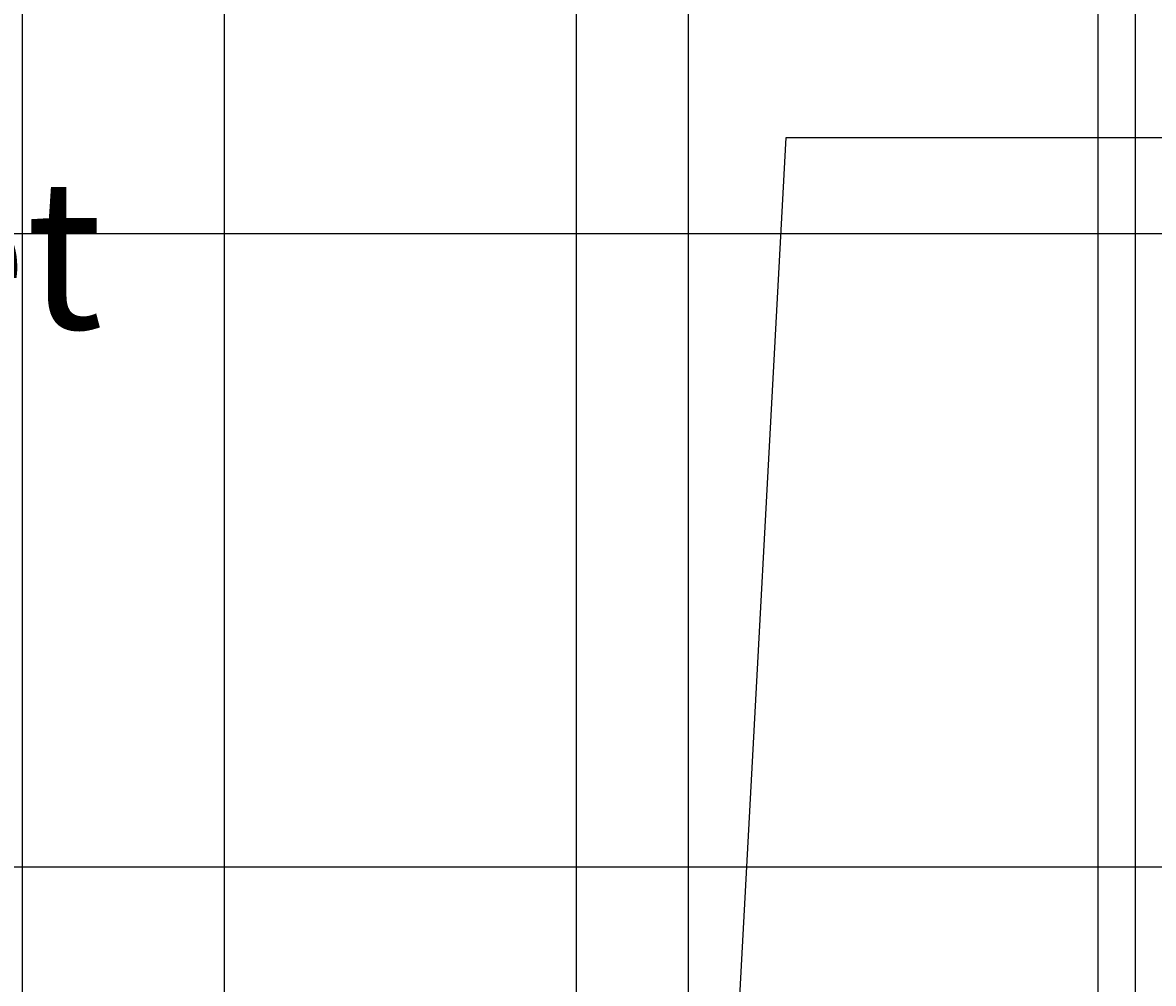
# Model space of a CAD drawing. Units: inches. Extents: x -12 to 334, y -10 to 186.
# Tile 25 of 77: x 58 to 88, y 135 to 160. Entities that reach past the tile are written whole.
import ezdxf
from ezdxf import colors
from ezdxf.entities.mleader import LeaderData, LeaderLine
from ezdxf.math import Vec2, Vec3

# ---------------------------------------------------------------- set-up
doc = ezdxf.new("R2010")
doc.units = ezdxf.units.IN
doc.header["$MEASUREMENT"] = 0
doc.layers.add('M-ANNO-TEXT', color=3, linetype='Continuous', lineweight=25)
doc.layers.add('M-DIMS', color=2, linetype='Continuous', lineweight=18)
doc.styles.get("Standard").update_dxf_attribs({"font": 'arial.ttf'})
doc.dimstyles.get("Standard").update_dxf_attribs({"dimtxt": 0.18, "dimasz": 0.18, "dimexe": 0.18, "dimexo": 0.0625, "dimgap": 0.09, "dimtad": 0, "dimtih": 1, "dimtoh": 1, "dimdec": 4, "dimzin": 0, "dimdsep": 46, "dimtxsty": 'Standard', "dimcen": 0.09, "dimadec": 0, "dimazin": 0, "dimtfac": 1, "dimtdec": 4, "dimtofl": 0, "dimtmove": 0, "dimatfit": 3, "dimfxl": 1, "dimtolj": 1, "dimtzin": 0, "dimarcsym": 0})

# ---------------------------------------------------------------- blocks, each defined once
blk = doc.blocks.new('*D3')
at = {"layer": 'Defpoints', "color": 0, "transparency": 16777216}
for p in [(58.1, 169.385), (32.1, 127.708), (58.1, 127.708)]:
    blk.add_point(p, dxfattribs=at)
at = {"layer": 'M-DIMS', "color": 0, "lineweight": -2, "transparency": 16777216}
for p, q in [((32.1, 127.77), (32.1, 169.565)), ((58.1, 127.77), (58.1, 169.565)), ((32.28, 169.385), (44.88, 169.385)), ((57.92, 169.385), (45.321, 169.385))]:
    blk.add_line(p, q, dxfattribs=at)
at = {"layer": 'M-DIMS', "color": 0, "transparency": 16777216}
for points in [[(32.28, 169.415), (32.28, 169.355), (32.1, 169.385)], [(57.92, 169.415), (57.92, 169.355), (58.1, 169.385)]]:
    blk.add_solid(points, dxfattribs=at)
at = {"layer": 'M-DIMS', "color": 0, "transparency": 16777216, "insert": (45.1, 169.385), "char_height": 0.18, "attachment_point": 5}
blk.add_mtext('\\A1;26', dxfattribs=at)
blk = doc.blocks.new('*D10')
at = {"layer": 'Defpoints', "color": 0, "transparency": 16777216}
for p in [(63.5, 169.385), (58.1, 127.708), (63.5, 109.058)]:
    blk.add_point(p, dxfattribs=at)
at = {"layer": 'M-DIMS', "color": 0, "lineweight": -2, "transparency": 16777216}
for p, q in [((58.1, 127.77), (58.1, 169.565)), ((63.5, 109.121), (63.5, 169.565)), ((58.28, 169.385), (60.547, 169.385)), ((63.32, 169.385), (61.054, 169.385))]:
    blk.add_line(p, q, dxfattribs=at)
at = {"layer": 'M-DIMS', "color": 0, "transparency": 16777216}
for points in [[(58.28, 169.415), (58.28, 169.355), (58.1, 169.385)], [(63.32, 169.415), (63.32, 169.355), (63.5, 169.385)]]:
    blk.add_solid(points, dxfattribs=at)
at = {"layer": 'M-DIMS', "color": 0, "transparency": 16777216, "insert": (60.8, 169.385), "char_height": 0.18, "attachment_point": 5}
blk.add_mtext('\\A1;5.4', dxfattribs=at)
blk = doc.blocks.new('*D11')
at = {"layer": 'Defpoints', "color": 0, "transparency": 16777216}
for p in [(72.924, 169.385), (63.5, 109.058), (72.924, 109.058)]:
    blk.add_point(p, dxfattribs=at)
at = {"layer": 'M-DIMS', "color": 0, "lineweight": -2, "transparency": 16777216}
for p, q in [((63.5, 109.121), (63.5, 169.565)), ((72.924, 109.121), (72.924, 169.565)), ((63.68, 169.385), (67.819, 169.385)), ((72.744, 169.385), (68.606, 169.385))]:
    blk.add_line(p, q, dxfattribs=at)
at = {"layer": 'M-DIMS', "color": 0, "transparency": 16777216}
for points in [[(63.68, 169.415), (63.68, 169.355), (63.5, 169.385)], [(72.744, 169.415), (72.744, 169.355), (72.924, 169.385)]]:
    blk.add_solid(points, dxfattribs=at)
at = {"layer": 'M-DIMS', "color": 0, "transparency": 16777216, "insert": (68.212, 169.385), "char_height": 0.18, "attachment_point": 5}
blk.add_mtext('\\A1;9.424', dxfattribs=at)
blk = doc.blocks.new('*D12')
at = {"layer": 'Defpoints', "color": 0, "transparency": 16777216}
for p in [(75.924, 169.385), (72.924, 109.058), (75.924, 109.058)]:
    blk.add_point(p, dxfattribs=at)
at = {"layer": 'M-DIMS', "color": 0, "lineweight": -2, "transparency": 16777216}
for p, q in [((72.924, 109.121), (72.924, 169.565)), ((75.924, 109.121), (75.924, 169.565)), ((73.104, 169.385), (74.275, 169.385)), ((75.744, 169.385), (74.573, 169.385))]:
    blk.add_line(p, q, dxfattribs=at)
at = {"layer": 'M-DIMS', "color": 0, "transparency": 16777216}
for points in [[(73.104, 169.415), (73.104, 169.355), (72.924, 169.385)], [(75.744, 169.415), (75.744, 169.355), (75.924, 169.385)]]:
    blk.add_solid(points, dxfattribs=at)
at = {"layer": 'M-DIMS', "color": 0, "transparency": 16777216, "insert": (74.424, 169.385), "char_height": 0.18, "attachment_point": 5}
blk.add_mtext('\\A1;3', dxfattribs=at)
blk = doc.blocks.new('*D13')
at = {"layer": 'Defpoints', "color": 0, "transparency": 16777216}
for p in [(86.888, 169.385), (75.924, 109.058), (86.888, 109.058)]:
    blk.add_point(p, dxfattribs=at)
at = {"layer": 'M-DIMS', "color": 0, "lineweight": -2, "transparency": 16777216}
for p, q in [((75.924, 109.121), (75.924, 169.565)), ((86.888, 109.121), (86.888, 169.565)), ((76.104, 169.385), (80.951, 169.385)), ((86.708, 169.385), (81.861, 169.385))]:
    blk.add_line(p, q, dxfattribs=at)
at = {"layer": 'M-DIMS', "color": 0, "transparency": 16777216}
for points in [[(76.104, 169.415), (76.104, 169.355), (75.924, 169.385)], [(86.708, 169.415), (86.708, 169.355), (86.888, 169.385)]]:
    blk.add_solid(points, dxfattribs=at)
at = {"layer": 'M-DIMS', "color": 0, "transparency": 16777216, "insert": (81.406, 169.385), "char_height": 0.18, "attachment_point": 5}
blk.add_mtext('\\A1;10.964', dxfattribs=at)
blk = doc.blocks.new('*D15')
at = {"layer": 'Defpoints', "color": 0, "transparency": 16777216}
for p in [(106.177, 169.385), (86.888, 109.058), (106.177, 102.896)]:
    blk.add_point(p, dxfattribs=at)
at = {"layer": 'M-DIMS', "color": 0, "lineweight": -2, "transparency": 16777216}
for p, q in [((86.888, 109.121), (86.888, 169.565)), ((106.177, 102.958), (106.177, 169.565)), ((87.068, 169.385), (96.147, 169.385)), ((105.997, 169.385), (96.918, 169.385))]:
    blk.add_line(p, q, dxfattribs=at)
at = {"layer": 'M-DIMS', "color": 0, "transparency": 16777216}
for points in [[(87.068, 169.415), (87.068, 169.355), (86.888, 169.385)], [(105.997, 169.415), (105.997, 169.355), (106.177, 169.385)]]:
    blk.add_solid(points, dxfattribs=at)
at = {"layer": 'M-DIMS', "color": 0, "transparency": 16777216, "insert": (96.532, 169.385), "char_height": 0.18, "attachment_point": 5}
blk.add_mtext('\\A1;19.29', dxfattribs=at)
blk = doc.blocks.new('*D22')
at = {"layer": 'Defpoints', "color": 0, "transparency": 16777216}
for p in [(190.342, 154.835), (-11.174, 137.887), (195.342, 137.887)]:
    blk.add_point(p, dxfattribs=at)
at = {"layer": 'M-DIMS', "color": 0, "lineweight": -2, "transparency": 16777216}
for p, q in [((190.28, 154.835), (-11.354, 154.835)), ((-11.174, 154.655), (-11.174, 146.543)), ((-11.174, 138.067), (-11.174, 146.179)), ((195.28, 137.887), (-11.354, 137.887))]:
    blk.add_line(p, q, dxfattribs=at)
at = {"layer": 'M-DIMS', "color": 0, "transparency": 16777216}
for points in [[(-11.204, 154.655), (-11.144, 154.655), (-11.174, 154.835)], [(-11.204, 138.067), (-11.144, 138.067), (-11.174, 137.887)]]:
    blk.add_solid(points, dxfattribs=at)
at = {"layer": 'M-DIMS', "color": 0, "transparency": 16777216, "insert": (-11.174, 146.361), "char_height": 0.18, "attachment_point": 5}
blk.add_mtext('\\A1;16.947', dxfattribs=at)
blk = doc.blocks.new('*D26')
at = {"layer": 'Defpoints', "color": 0, "transparency": 16777216}
for p in [(87.888, 169.385), (87.888, 56.321), (58.1, 33.675)]:
    blk.add_point(p, dxfattribs=at)
at = {"layer": 'M-DIMS', "color": 0, "lineweight": -2, "transparency": 16777216}
for p, q in [((58.1, 33.738), (58.1, 169.565)), ((87.888, 56.383), (87.888, 169.565)), ((58.28, 169.385), (72.599, 169.385)), ((87.708, 169.385), (73.389, 169.385))]:
    blk.add_line(p, q, dxfattribs=at)
at = {"layer": 'M-DIMS', "color": 0, "transparency": 16777216}
for points in [[(58.28, 169.415), (58.28, 169.355), (58.1, 169.385)], [(87.708, 169.415), (87.708, 169.355), (87.888, 169.385)]]:
    blk.add_solid(points, dxfattribs=at)
at = {"layer": 'M-DIMS', "color": 0, "transparency": 16777216, "insert": (72.994, 169.385), "char_height": 0.18, "attachment_point": 5}
blk.add_mtext('\\A1;29.79', dxfattribs=at)

msp = doc.modelspace()

# ---------------------------------------------------------------- texts
at = {"layer": 'M-ANNO-TEXT', "insert": (31.1039, 156.2953), "char_height": 4, "attachment_point": 1}
msp.add_mtext_dynamic_manual_height_columns('Steam inlet', width=36.185701, gutter_width=1, heights=[0], dxfattribs=at)

# ---------------------------------------------------------------- dimensions: what is measured, and where the dimension line sits
at = {"layer": 'M-DIMS'}
for base, p1, p2, override, picture, middle in [((58.1002, 169.3845), (32.1002, 127.7078), (58.1002, 127.7078), {"dimdec": 0, "dimlfac": 1, "dimrnd": 0, "dimzin": 0, "dimdsep": 46, "dimlunit": 2}, '*D3', (45.1002, 169.3845)), ((63.5, 169.3845), (58.1002, 127.7078), (63.5, 109.0583), {"dimdec": 1, "dimlfac": 1, "dimrnd": 0, "dimzin": 0, "dimdsep": 46, "dimlunit": 2}, '*D10', (60.8001, 169.3845)), ((87.8879, 169.3845), (58.1002, 33.6752), (87.8879, 56.3205), {"dimdec": 2, "dimlfac": 1, "dimrnd": 0, "dimzin": 0, "dimdsep": 46, "dimlunit": 2}, '*D26', (72.9941, 169.3845)), ((72.9244, 169.3845), (63.5, 109.0583), (72.9244, 109.0583), {"dimdec": 3, "dimlfac": 1, "dimrnd": 0, "dimzin": 0, "dimdsep": 46, "dimlunit": 2}, '*D11', (68.2122, 169.3845)), ((75.9244, 169.3845), (72.9244, 109.0583), (75.9244, 109.0583), {"dimdec": 0, "dimlfac": 1, "dimrnd": 0, "dimzin": 0, "dimdsep": 46, "dimlunit": 2}, '*D12', (74.4244, 169.3845)), ((86.887907, 169.384532), (75.924407, 109.05834), (86.887907, 109.05834), {"dimdec": 3, "dimlfac": 1, "dimrnd": 0, "dimzin": 0, "dimdsep": 46, "dimlunit": 2}, '*D13', (81.406157, 169.384532)), ((106.1771, 169.3845), (86.8879, 109.0583), (106.1771, 102.8958), {"dimdec": 2, "dimlfac": 1, "dimrnd": 0, "dimzin": 0, "dimdsep": 46, "dimlunit": 2}, '*D15', (96.5325, 169.3845))]:
    dim = msp.add_linear_dim(base=base, p1=p1, p2=p2, dimstyle='Standard', override=override, dxfattribs=at)
    dim.commit()
    dim.dimension.update_dxf_attribs({"geometry": picture, "text_midpoint": middle})
dim = msp.add_linear_dim(base=(-11.1736, 137.8871), p1=(190.3421, 154.8345), p2=(195.3421, 137.8871), angle=90, dimstyle='Standard', override={"dimdec": 3, "dimlfac": 1, "dimrnd": 0, "dimzin": 0, "dimdsep": 46, "dimlunit": 2}, dxfattribs=at)
dim.commit()
dim.dimension.update_dxf_attribs({"geometry": '*D22', "text_midpoint": (-11.1735, 146.3608)})

# ---------------------------------------------------------------- leaders
at = {"layer": 'M-ANNO-TEXT'}
ml = msp.add_multileader_mtext('Standard', dxfattribs=at)
ml.set_content('Tube plate', color=256)
ml.set_leader_properties()
ml.build(insert=Vec2(0, 0))
ml.multileader.update_dxf_attribs({"dogleg_length": 0.36, "arrow_head_size": 0.7})
ctx = ml.context
ctx.base_point, ctx.arrow_head_size, ctx.landing_gap_size, ctx.plane_origin = Vec3(95.9742, 157.4218), 0.7, 0.09, Vec3(31.4743, 171.7024)
notes = []
notes.append((ctx, [(0, (1, 1, 0), (78.5354, 157.4218), (1, 0), 17.4388, [(0, [(75.9244, 109.0583)], 0, [])])]))
ctx.mtext.insert, ctx.mtext.flow_direction = Vec3(96.0642, 159.9771), 5
for ctx, leaders in notes:
    for number, flags, end, landing, length, lines in leaders:
        leader = LeaderData()
        leader.index, (leader.has_last_leader_line, leader.has_dogleg_vector, leader.attachment_direction) = number, flags
        leader.last_leader_point, leader.dogleg_vector, leader.dogleg_length = Vec3(end), Vec3(landing), length
        for number, points, colour, breaks in lines:
            line = LeaderLine()
            line.index, line.vertices, line.color, line.breaks = number, Vec3.list(points), colors.encode_raw_color(colour), breaks
            leader.lines.append(line)
        ctx.leaders.append(leader)

doc.saveas('drawing.dxf')
